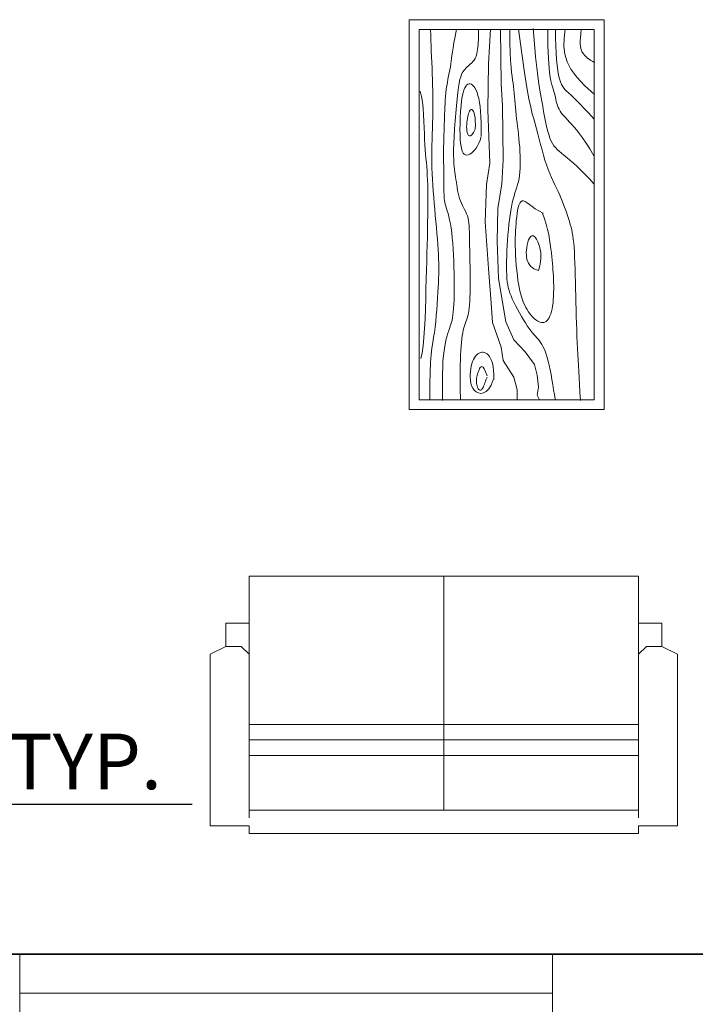
# Model space of a CAD drawing. Units: inches. Extents: x 1265 to 2734, y 1741 to 2595.
# Tile 5 of 10: x 2573 to 2634, y 1988 to 2076. Entities that reach past the tile are written whole.
import ezdxf

# ---------------------------------------------------------------- set-up
doc = ezdxf.new("R2010")
doc.units = ezdxf.units.IN
doc.header["$LTSCALE"] = 0.1
for name, color, linetype, lineweight in [('A-ANNO-DIMS', 2, 'Continuous', 18), ('A-GLAZ', 4, 'Continuous', 18), ('A-WALL', 7, 'Continuous', 35), ('Furniture', 8, 'Continuous', 15)]:
    doc.layers.add(name, color=color, linetype=linetype, lineweight=lineweight)
doc.styles.get("Standard").update_dxf_attribs({"font": 'arial.ttf', "height": 5})
doc.dimstyles.new('ISO-25', dxfattribs={"dimtxt": 5, "dimasz": 2.5, "dimexe": 1.25, "dimexo": 0.625, "dimtad": 1, "dimlunit": 3, "dimtxsty": 'Standard', "dimcen": 2.5, "dimadec": 0, "dimazin": 0, "dimtfac": 1, "dimtmove": 0, "dimatfit": 3, "dimfxl": 1, "dimarcsym": 0})

# ---------------------------------------------------------------- blocks, each defined once
blk = doc.blocks.new('WINDOW-48IN')
for p, q in [((0, 9), (0, 0)), ((48, 9), (0, 9)), ((48, 9), (48, 0)), ((48, 5.5), (0, 5.5)), ((48, 3.5), (0, 3.5)), ((0, 0), (48, 0))]:
    blk.add_line(p, q)
blk = doc.blocks.new('*D34')
at = {"layer": 'A-ANNO-DIMS', "color": 0, "lineweight": -2, "transparency": 16777216}
for p, q in [((2441.102, 2014.032), (2441.102, 2004.407)), ((2501.102, 2014.032), (2501.102, 2004.407)), ((2443.602, 2005.657), (2498.602, 2005.657)), ((2501.102, 2005.657), (2588.642, 2005.657))]:
    blk.add_line(p, q, dxfattribs=at)
at = {"layer": 'A-ANNO-DIMS', "color": 0, "lineweight": 100, "transparency": 16777216}
for points in [[(2443.602, 2006.073), (2443.602, 2005.24), (2441.102, 2005.657)], [(2498.602, 2006.073), (2498.602, 2005.24), (2501.102, 2005.657)]]:
    blk.add_solid(points, dxfattribs=at)
at = {"layer": 'Defpoints', "color": 0, "lineweight": 100, "transparency": 16777216}
for p in [(2441.102, 2014.657), (2501.102, 2014.657), (2501.102, 2005.657)]:
    blk.add_point(p, dxfattribs=at)
at = {"layer": 'A-ANNO-DIMS', "color": 0, "transparency": 16777216, "insert": (2546.122, 2008.869), "char_height": 5, "attachment_point": 5}
blk.add_mtext('DOUBLE DOOR 5\'-0" TYP.', dxfattribs=at)

msp = doc.modelspace()

# ---------------------------------------------------------------- linework, layer by layer
at = {"layer": 'A-WALL'}
msp.add_line((2514.602, 1992.157), (2679.602, 1992.157), dxfattribs=at)
at = {"layer": 'Furniture'}
for p, q in [((2608.19, 2041.186), (2608.19, 2076.268)), ((2608.19, 2076.268), (2625.731, 2076.268)), ((2625.731, 2076.268), (2625.731, 2041.186)), ((2609.067, 2042.063), (2609.067, 2075.391)), ((2609.067, 2075.391), (2624.854, 2075.391)), ((2610.115, 2075.344), (2610.119, 2074.885)), ((2612.454, 2075.404), (2612.315, 2074.746)), ((2614.432, 2075.344), (2614.421, 2074.614)), ((2615.511, 2075.404), (2615.332, 2072.285)), ((2616.411, 2075.344), (2616.471, 2070.485)), ((2617.25, 2075.344), (2617.258, 2074.223)), ((2618.03, 2075.404), (2618.322, 2073.226)), ((2619.349, 2075.464), (2619.459, 2074.082)), ((2620.668, 2075.344), (2620.682, 2073.911)), ((2621.347, 2075.424), (2621.354, 2074.634)), ((2622.227, 2075.404), (2622.126, 2074.593)), ((2623.666, 2075.404), (2623.627, 2075.005)), ((2624.854, 2075.391), (2624.854, 2042.063)), ((2610.119, 2074.885), (2610.13, 2074.409)), ((2610.13, 2074.409), (2610.146, 2073.92)), ((2612.315, 2074.746), (2612.209, 2074.2)), ((2614.421, 2074.614), (2614.39, 2074.03)), ((2621.354, 2074.634), (2621.374, 2073.913)), ((2622.126, 2074.593), (2622.108, 2073.853)), ((2623.6, 2074.659), (2623.587, 2074.36)), ((2623.627, 2075.005), (2623.6, 2074.659)), ((2610.146, 2073.92), (2610.167, 2073.421)), ((2612.131, 2073.747), (2612.074, 2073.372)), ((2612.209, 2074.2), (2612.131, 2073.747)), ((2614.342, 2073.573), (2614.279, 2073.223)), ((2614.39, 2074.03), (2614.342, 2073.573)), ((2617.258, 2074.223), (2617.28, 2073.312)), ((2619.459, 2074.082), (2619.563, 2072.929)), ((2620.682, 2073.911), (2620.722, 2072.779)), ((2621.374, 2073.913), (2621.407, 2073.259)), ((2622.108, 2073.853), (2622.192, 2073.159)), ((2623.587, 2074.36), (2623.589, 2074.101)), ((2623.589, 2074.101), (2623.607, 2073.877)), ((2623.607, 2073.877), (2623.643, 2073.681)), ((2623.643, 2073.681), (2623.697, 2073.507)), ((2623.697, 2073.507), (2623.771, 2073.349)), ((2610.167, 2073.421), (2610.19, 2072.916)), ((2610.19, 2072.916), (2610.214, 2072.406)), ((2611.998, 2072.78), (2611.968, 2072.529)), ((2612.032, 2073.055), (2611.998, 2072.78)), ((2612.074, 2073.372), (2612.032, 2073.055)), ((2614.022, 2072.618), (2613.923, 2072.5)), ((2614.116, 2072.765), (2614.022, 2072.618)), ((2614.202, 2072.96), (2614.116, 2072.765)), ((2614.279, 2073.223), (2614.202, 2072.96)), ((2617.28, 2073.312), (2617.313, 2072.581)), ((2618.322, 2073.226), (2618.572, 2071.505)), ((2619.563, 2072.929), (2619.663, 2071.97)), ((2620.722, 2072.779), (2620.782, 2071.905)), ((2621.407, 2073.259), (2621.451, 2072.671)), ((2621.451, 2072.671), (2621.505, 2072.148)), ((2622.192, 2073.159), (2622.399, 2072.487)), ((2623.771, 2073.349), (2623.865, 2073.202)), ((2623.865, 2073.202), (2623.978, 2073.065)), ((2623.978, 2073.065), (2624.105, 2072.936)), ((2624.105, 2072.936), (2624.245, 2072.815)), ((2624.245, 2072.815), (2624.394, 2072.702)), ((2624.394, 2072.702), (2624.549, 2072.597)), ((2610.214, 2072.406), (2610.238, 2071.897)), ((2610.238, 2071.897), (2610.26, 2071.39)), ((2611.843, 2071.768), (2611.789, 2071.495)), ((2611.892, 2072.032), (2611.843, 2071.768)), ((2611.934, 2072.285), (2611.892, 2072.032)), ((2611.968, 2072.529), (2611.934, 2072.285)), ((2613.212, 2071.826), (2613.123, 2071.725)), ((2613.307, 2071.922), (2613.212, 2071.826)), ((2613.406, 2072.015), (2613.307, 2071.922)), ((2613.508, 2072.107), (2613.406, 2072.015)), ((2613.612, 2072.199), (2613.508, 2072.107)), ((2613.716, 2072.293), (2613.612, 2072.199)), ((2613.82, 2072.393), (2613.716, 2072.293)), ((2613.923, 2072.5), (2613.82, 2072.393)), ((2615.332, 2072.285), (2615.272, 2068.145)), ((2617.313, 2072.581), (2617.354, 2072)), ((2617.354, 2072), (2617.4, 2071.536)), ((2619.663, 2071.97), (2619.76, 2071.174)), ((2620.782, 2071.905), (2620.856, 2071.246)), ((2621.505, 2072.148), (2621.569, 2071.688)), ((2622.399, 2072.487), (2622.75, 2071.812)), ((2622.75, 2071.812), (2623.264, 2071.11)), ((2624.549, 2072.597), (2624.707, 2072.498)), ((2624.707, 2072.498), (2624.865, 2072.405)), ((2610.26, 2071.39), (2610.279, 2070.888)), ((2610.279, 2070.888), (2610.294, 2070.392)), ((2611.676, 2070.921), (2611.62, 2070.623)), ((2611.733, 2071.212), (2611.676, 2070.921)), ((2611.789, 2071.495), (2611.733, 2071.212)), ((2612.755, 2070.879), (2612.69, 2070.568)), ((2612.821, 2071.129), (2612.755, 2070.879)), ((2612.89, 2071.327), (2612.821, 2071.129)), ((2612.963, 2071.485), (2612.89, 2071.327)), ((2613.04, 2071.614), (2612.963, 2071.485)), ((2613.123, 2071.725), (2613.04, 2071.614)), ((2617.4, 2071.536), (2617.448, 2071.16)), ((2617.448, 2071.16), (2617.496, 2070.84)), ((2618.572, 2071.505), (2618.786, 2070.171)), ((2619.76, 2071.174), (2619.853, 2070.507)), ((2620.856, 2071.246), (2620.939, 2070.76)), ((2621.569, 2071.688), (2621.642, 2071.289)), ((2621.642, 2071.289), (2621.722, 2070.95)), ((2621.722, 2070.95), (2621.81, 2070.668)), ((2623.264, 2071.11), (2623.962, 2070.356)), ((2610.294, 2070.392), (2610.306, 2069.899)), ((2611.524, 2070.005), (2611.487, 2069.688)), ((2611.569, 2070.317), (2611.524, 2070.005)), ((2611.62, 2070.623), (2611.569, 2070.317)), ((2612.627, 2070.183), (2612.563, 2069.715)), ((2612.69, 2070.568), (2612.627, 2070.183)), ((2613.189, 2070.139), (2613.107, 2069.933)), ((2613.277, 2070.293), (2613.189, 2070.139)), ((2613.371, 2070.401), (2613.277, 2070.293)), ((2613.47, 2070.467), (2613.371, 2070.401)), ((2613.573, 2070.495), (2613.47, 2070.467)), ((2613.679, 2070.49), (2613.573, 2070.495)), ((2613.788, 2070.451), (2613.679, 2070.49)), ((2613.896, 2070.377), (2613.788, 2070.451)), ((2614.003, 2070.268), (2613.896, 2070.377)), ((2614.106, 2070.123), (2614.003, 2070.268)), ((2614.204, 2069.94), (2614.106, 2070.123)), ((2616.471, 2070.485), (2616.591, 2068.505)), ((2617.496, 2070.84), (2617.54, 2070.545)), ((2617.54, 2070.545), (2617.578, 2070.25)), ((2617.578, 2070.25), (2617.611, 2069.949)), ((2618.786, 2070.171), (2618.97, 2069.156)), ((2619.853, 2070.507), (2619.943, 2069.936)), ((2620.939, 2070.76), (2621.024, 2070.405)), ((2621.024, 2070.405), (2621.107, 2070.137)), ((2621.107, 2070.137), (2621.183, 2069.915)), ((2621.81, 2070.668), (2621.905, 2070.437)), ((2621.905, 2070.437), (2622.005, 2070.247)), ((2622.005, 2070.247), (2622.113, 2070.091)), ((2622.113, 2070.091), (2622.226, 2069.959)), ((2622.226, 2069.959), (2622.344, 2069.843)), ((2623.962, 2070.356), (2624.865, 2069.525)), ((2609.156, 2069.825), (2609.275, 2069.365)), ((2609.275, 2069.365), (2609.365, 2068.85)), ((2610.306, 2069.899), (2610.314, 2069.41)), ((2610.314, 2069.41), (2610.318, 2068.921)), ((2611.457, 2069.366), (2611.433, 2069.043)), ((2611.487, 2069.688), (2611.457, 2069.366)), ((2612.5, 2069.158), (2612.437, 2068.529)), ((2612.563, 2069.715), (2612.5, 2069.158)), ((2612.964, 2069.351), (2612.903, 2068.965)), ((2613.032, 2069.672), (2612.964, 2069.351)), ((2613.107, 2069.933), (2613.032, 2069.672)), ((2614.295, 2069.72), (2614.204, 2069.94)), ((2614.377, 2069.46), (2614.295, 2069.72)), ((2614.449, 2069.161), (2614.377, 2069.46)), ((2614.51, 2068.82), (2614.449, 2069.161)), ((2617.611, 2069.949), (2617.641, 2069.643)), ((2617.641, 2069.643), (2617.667, 2069.331)), ((2617.667, 2069.331), (2617.693, 2069.015)), ((2618.97, 2069.156), (2619.13, 2068.39)), ((2619.943, 2069.936), (2620.032, 2069.428)), ((2620.032, 2069.428), (2620.118, 2068.95)), ((2621.183, 2069.915), (2621.246, 2069.703)), ((2621.246, 2069.703), (2621.299, 2069.494)), ((2621.299, 2069.494), (2621.345, 2069.29)), ((2621.345, 2069.29), (2621.388, 2069.091)), ((2621.388, 2069.091), (2621.431, 2068.899)), ((2622.344, 2069.843), (2622.468, 2069.734)), ((2622.468, 2069.734), (2622.597, 2069.625)), ((2622.597, 2069.625), (2622.732, 2069.506)), ((2622.732, 2069.506), (2622.885, 2069.364)), ((2622.885, 2069.364), (2623.067, 2069.187)), ((2623.067, 2069.187), (2623.29, 2068.963)), ((2609.365, 2068.85), (2609.431, 2068.296)), ((2609.431, 2068.296), (2609.478, 2067.717)), ((2610.318, 2068.434), (2610.314, 2067.945)), ((2610.318, 2068.921), (2610.318, 2068.434)), ((2611.399, 2068.397), (2611.386, 2068.077)), ((2611.414, 2068.719), (2611.399, 2068.397)), ((2611.433, 2069.043), (2611.414, 2068.719)), ((2612.437, 2068.529), (2612.377, 2067.852)), ((2612.851, 2068.514), (2612.809, 2068.012)), ((2612.903, 2068.965), (2612.851, 2068.514)), ((2614.561, 2068.435), (2614.51, 2068.82)), ((2614.601, 2068.006), (2614.561, 2068.435)), ((2616.591, 2068.505), (2616.651, 2063.646)), ((2617.693, 2069.015), (2617.72, 2068.693)), ((2617.72, 2068.693), (2617.748, 2068.367)), ((2617.748, 2068.367), (2617.78, 2068.035)), ((2619.13, 2068.39), (2619.271, 2067.805)), ((2620.118, 2068.95), (2620.204, 2068.475)), ((2620.204, 2068.475), (2620.29, 2068.004)), ((2621.431, 2068.899), (2621.478, 2068.713)), ((2621.478, 2068.713), (2621.533, 2068.535)), ((2621.533, 2068.535), (2621.597, 2068.365)), ((2621.597, 2068.365), (2621.676, 2068.204)), ((2621.676, 2068.204), (2621.768, 2068.05)), ((2623.29, 2068.963), (2623.567, 2068.677)), ((2623.567, 2068.677), (2623.911, 2068.318)), ((2623.911, 2068.318), (2624.332, 2067.871)), ((2609.478, 2067.717), (2609.511, 2067.13)), ((2610.305, 2067.455), (2610.292, 2066.963)), ((2610.314, 2067.945), (2610.305, 2067.455)), ((2611.364, 2067.455), (2611.353, 2067.155)), ((2611.375, 2067.763), (2611.364, 2067.455)), ((2611.386, 2068.077), (2611.375, 2067.763)), ((2612.377, 2067.852), (2612.321, 2067.151)), ((2612.778, 2067.479), (2612.758, 2066.934)), ((2612.809, 2068.012), (2612.778, 2067.479)), ((2613.424, 2067.388), (2613.395, 2067.21)), ((2613.457, 2067.554), (2613.424, 2067.388)), ((2613.493, 2067.705), (2613.457, 2067.554)), ((2613.531, 2067.838), (2613.493, 2067.705)), ((2613.572, 2067.951), (2613.531, 2067.838)), ((2613.614, 2068.043), (2613.572, 2067.951)), ((2613.659, 2068.113), (2613.614, 2068.043)), ((2613.706, 2068.159), (2613.659, 2068.113)), ((2613.756, 2068.181), (2613.706, 2068.159)), ((2613.808, 2068.176), (2613.756, 2068.181)), ((2613.863, 2068.145), (2613.808, 2068.176)), ((2613.92, 2068.085), (2613.863, 2068.145)), ((2613.976, 2067.992), (2613.92, 2068.085)), ((2614.03, 2067.859), (2613.976, 2067.992)), ((2614.076, 2067.68), (2614.03, 2067.859)), ((2614.113, 2067.452), (2614.076, 2067.68)), ((2614.137, 2067.167), (2614.113, 2067.452)), ((2614.633, 2067.53), (2614.601, 2068.006)), ((2614.655, 2067.006), (2614.633, 2067.53)), ((2615.272, 2068.145), (2615.451, 2063.346)), ((2617.78, 2068.035), (2617.816, 2067.699)), ((2617.816, 2067.699), (2617.855, 2067.358)), ((2617.855, 2067.358), (2617.897, 2067.012)), ((2619.271, 2067.805), (2619.401, 2067.332)), ((2619.401, 2067.332), (2619.524, 2066.901)), ((2620.29, 2068.004), (2620.376, 2067.542)), ((2620.376, 2067.542), (2620.464, 2067.097)), ((2621.768, 2068.05), (2621.875, 2067.897)), ((2621.875, 2067.897), (2621.996, 2067.744)), ((2621.996, 2067.744), (2622.131, 2067.587)), ((2622.131, 2067.587), (2622.282, 2067.422)), ((2622.282, 2067.422), (2622.447, 2067.246)), ((2624.332, 2067.871), (2624.845, 2067.325)), ((2609.511, 2067.13), (2609.535, 2066.55)), ((2609.535, 2066.55), (2609.555, 2065.992)), ((2610.275, 2066.468), (2610.258, 2065.969)), ((2610.292, 2066.963), (2610.275, 2066.468)), ((2611.328, 2066.558), (2611.317, 2066.249)), ((2611.341, 2066.858), (2611.328, 2066.558)), ((2611.353, 2067.155), (2611.341, 2066.858)), ((2612.272, 2066.447), (2612.232, 2065.764)), ((2612.321, 2067.151), (2612.272, 2066.447)), ((2612.758, 2066.934), (2612.752, 2066.396)), ((2613.359, 2066.834), (2613.354, 2066.644)), ((2613.354, 2066.644), (2613.36, 2066.456)), ((2613.374, 2067.024), (2613.359, 2066.834)), ((2613.36, 2066.456), (2613.378, 2066.276)), ((2613.395, 2067.21), (2613.374, 2067.024)), ((2614.132, 2066.406), (2614.144, 2066.82)), ((2614.144, 2066.82), (2614.137, 2067.167)), ((2614.668, 2066.432), (2614.655, 2067.006)), ((2614.672, 2065.806), (2614.668, 2066.432)), ((2617.897, 2067.012), (2617.94, 2066.659)), ((2617.94, 2066.659), (2617.983, 2066.301)), ((2619.524, 2066.901), (2619.645, 2066.455)), ((2619.645, 2066.455), (2619.767, 2065.991)), ((2620.464, 2067.097), (2620.555, 2066.676)), ((2620.555, 2066.676), (2620.648, 2066.284)), ((2622.447, 2067.246), (2622.627, 2067.056)), ((2622.627, 2067.056), (2622.822, 2066.846)), ((2622.822, 2066.846), (2623.034, 2066.609)), ((2623.034, 2066.609), (2623.267, 2066.332)), ((2609.555, 2065.992), (2609.575, 2065.471)), ((2610.258, 2065.969), (2610.241, 2065.468)), ((2611.297, 2065.587), (2611.289, 2065.221)), ((2611.306, 2065.928), (2611.297, 2065.587)), ((2611.317, 2066.249), (2611.306, 2065.928)), ((2612.232, 2065.764), (2612.202, 2065.126)), ((2612.752, 2066.396), (2612.76, 2065.885)), ((2612.76, 2065.885), (2612.783, 2065.418)), ((2613.378, 2066.276), (2613.409, 2066.107)), ((2613.409, 2066.107), (2613.456, 2065.963)), ((2613.456, 2065.963), (2613.519, 2065.857)), ((2613.519, 2065.857), (2613.6, 2065.805)), ((2613.6, 2065.805), (2613.7, 2065.819)), ((2613.7, 2065.819), (2613.821, 2065.914)), ((2613.821, 2065.914), (2613.965, 2066.105)), ((2613.965, 2066.105), (2614.132, 2066.406)), ((2614.574, 2065.428), (2614.672, 2065.746)), ((2617.983, 2066.301), (2618.024, 2065.936)), ((2618.024, 2065.936), (2618.064, 2065.565)), ((2618.064, 2065.565), (2618.1, 2065.186)), ((2619.767, 2065.991), (2619.89, 2065.514)), ((2620.648, 2066.284), (2620.746, 2065.928)), ((2620.746, 2065.928), (2620.848, 2065.616)), ((2620.848, 2065.616), (2620.956, 2065.35)), ((2623.267, 2066.332), (2623.521, 2066.007)), ((2623.521, 2066.007), (2623.8, 2065.622)), ((2623.8, 2065.622), (2624.105, 2065.167)), ((2609.575, 2065.471), (2609.601, 2064.999)), ((2609.601, 2064.999), (2609.63, 2064.569)), ((2610.227, 2064.964), (2610.216, 2064.458)), ((2610.241, 2065.468), (2610.227, 2064.964)), ((2611.284, 2064.826), (2611.282, 2064.398)), ((2611.289, 2065.221), (2611.284, 2064.826)), ((2612.202, 2065.126), (2612.184, 2064.556)), ((2612.783, 2065.418), (2612.823, 2065.016)), ((2612.823, 2065.016), (2612.881, 2064.693)), ((2612.881, 2064.693), (2612.954, 2064.446)), ((2614.068, 2064.516), (2614.206, 2064.693)), ((2614.206, 2064.693), (2614.338, 2064.903)), ((2614.338, 2064.903), (2614.462, 2065.147)), ((2614.462, 2065.147), (2614.574, 2065.428)), ((2618.1, 2065.186), (2618.131, 2064.8)), ((2618.131, 2064.8), (2618.156, 2064.412)), ((2619.89, 2065.514), (2620.015, 2065.032)), ((2620.015, 2065.032), (2620.143, 2064.552)), ((2620.956, 2065.35), (2621.073, 2065.125)), ((2621.073, 2065.125), (2621.201, 2064.93)), ((2621.201, 2064.93), (2621.344, 2064.757)), ((2621.344, 2064.757), (2621.504, 2064.594)), ((2624.105, 2065.167), (2624.439, 2064.632)), ((2609.63, 2064.569), (2609.662, 2064.171)), ((2609.662, 2064.171), (2609.695, 2063.793)), ((2609.695, 2063.793), (2609.729, 2063.426)), ((2610.216, 2064.458), (2610.212, 2063.948)), ((2610.212, 2063.948), (2610.215, 2063.436)), ((2611.282, 2064.398), (2611.282, 2063.945)), ((2611.282, 2063.945), (2611.284, 2063.479)), ((2612.184, 2064.556), (2612.179, 2064.071)), ((2612.179, 2064.071), (2612.187, 2063.663)), ((2612.954, 2064.446), (2613.042, 2064.268)), ((2613.042, 2064.268), (2613.143, 2064.152)), ((2613.143, 2064.152), (2613.255, 2064.091)), ((2613.255, 2064.091), (2613.377, 2064.078)), ((2613.377, 2064.078), (2613.507, 2064.105)), ((2613.507, 2064.105), (2613.643, 2064.166)), ((2613.643, 2064.166), (2613.783, 2064.254)), ((2613.783, 2064.254), (2613.926, 2064.371)), ((2613.926, 2064.371), (2614.068, 2064.516)), ((2618.156, 2064.412), (2618.175, 2064.024)), ((2618.175, 2064.024), (2618.185, 2063.642)), ((2620.143, 2064.552), (2620.273, 2064.081)), ((2620.273, 2064.081), (2620.408, 2063.627)), ((2621.504, 2064.594), (2621.684, 2064.434)), ((2621.684, 2064.434), (2621.887, 2064.266)), ((2621.887, 2064.266), (2622.117, 2064.081)), ((2622.117, 2064.081), (2622.375, 2063.871)), ((2622.375, 2063.871), (2622.659, 2063.631)), ((2624.439, 2064.632), (2624.805, 2064.006)), ((2609.729, 2063.426), (2609.761, 2063.057)), ((2609.761, 2063.057), (2609.79, 2062.678)), ((2610.215, 2063.436), (2610.227, 2062.921)), ((2610.227, 2062.921), (2610.247, 2062.403)), ((2611.284, 2063.479), (2611.287, 2063.011)), ((2611.287, 2063.011), (2611.291, 2062.553)), ((2612.187, 2063.663), (2612.204, 2063.32)), ((2612.204, 2063.32), (2612.229, 2063.029)), ((2612.229, 2063.029), (2612.259, 2062.776)), ((2615.451, 2063.346), (2615.152, 2061.427)), ((2616.651, 2063.646), (2616.531, 2061.486)), ((2618.176, 2062.912), (2618.154, 2062.573)), ((2618.185, 2063.27), (2618.176, 2062.912)), ((2618.185, 2063.642), (2618.185, 2063.27)), ((2620.408, 2063.627), (2620.548, 2063.196)), ((2620.548, 2063.196), (2620.693, 2062.795)), ((2622.659, 2063.631), (2622.968, 2063.362)), ((2622.968, 2063.362), (2623.3, 2063.059)), ((2623.3, 2063.059), (2623.652, 2062.723)), ((2609.79, 2062.678), (2609.815, 2062.276)), ((2609.815, 2062.276), (2609.835, 2061.844)), ((2610.247, 2062.403), (2610.275, 2061.881)), ((2611.291, 2062.553), (2611.296, 2062.115)), ((2611.296, 2062.115), (2611.3, 2061.709)), ((2612.259, 2062.776), (2612.293, 2062.548)), ((2612.293, 2062.548), (2612.329, 2062.333)), ((2612.329, 2062.333), (2612.364, 2062.116)), ((2612.364, 2062.116), (2612.396, 2061.889)), ((2618.12, 2062.256), (2618.072, 2061.965)), ((2618.154, 2062.573), (2618.12, 2062.256)), ((2620.693, 2062.795), (2620.842, 2062.42)), ((2620.842, 2062.42), (2620.994, 2062.067)), ((2620.994, 2062.067), (2621.146, 2061.733)), ((2623.652, 2062.723), (2624.021, 2062.35)), ((2624.021, 2062.35), (2624.406, 2061.938)), ((2609.835, 2061.844), (2609.85, 2061.38)), ((2609.85, 2061.38), (2609.859, 2060.886)), ((2610.275, 2061.881), (2610.309, 2061.355)), ((2610.309, 2061.355), (2610.348, 2060.825)), ((2611.3, 2061.709), (2611.304, 2061.347)), ((2611.304, 2061.347), (2611.308, 2061.035)), ((2612.396, 2061.889), (2612.428, 2061.65)), ((2612.428, 2061.65), (2612.461, 2061.405)), ((2612.461, 2061.405), (2612.497, 2061.155)), ((2612.497, 2061.155), (2612.539, 2060.905)), ((2615.152, 2061.427), (2615.032, 2058.067)), ((2616.531, 2061.486), (2616.171, 2059.267)), ((2617.867, 2061.185), (2617.787, 2060.934)), ((2617.943, 2061.436), (2617.867, 2061.185)), ((2618.012, 2061.694), (2617.943, 2061.436)), ((2618.072, 2061.965), (2618.012, 2061.694)), ((2621.146, 2061.733), (2621.299, 2061.412)), ((2621.299, 2061.412), (2621.449, 2061.1)), ((2621.449, 2061.1), (2621.596, 2060.793)), ((2624.406, 2061.938), (2624.805, 2061.486)), ((2609.859, 2060.886), (2609.864, 2060.363)), ((2609.864, 2060.363), (2609.865, 2059.812)), ((2610.348, 2060.825), (2610.391, 2060.291)), ((2610.391, 2060.291), (2610.437, 2059.752)), ((2611.308, 2061.035), (2611.312, 2060.769)), ((2611.312, 2060.769), (2611.318, 2060.541)), ((2611.318, 2060.541), (2611.328, 2060.342)), ((2611.328, 2060.342), (2611.343, 2060.163)), ((2612.539, 2060.905), (2612.587, 2060.658)), ((2612.587, 2060.658), (2612.645, 2060.418)), ((2612.645, 2060.418), (2612.713, 2060.187)), ((2617.621, 2060.401), (2617.54, 2060.107)), ((2617.704, 2060.675), (2617.621, 2060.401)), ((2617.787, 2060.934), (2617.704, 2060.675)), ((2621.596, 2060.793), (2621.737, 2060.487)), ((2621.737, 2060.487), (2621.873, 2060.178)), ((2609.865, 2059.812), (2609.862, 2059.235)), ((2610.437, 2059.752), (2610.485, 2059.207)), ((2611.343, 2060.163), (2611.365, 2059.997)), ((2611.365, 2059.997), (2611.395, 2059.834)), ((2611.395, 2059.834), (2611.434, 2059.667)), ((2611.434, 2059.667), (2611.484, 2059.487)), ((2611.484, 2059.487), (2611.544, 2059.29)), ((2612.713, 2060.187), (2612.794, 2059.968)), ((2612.794, 2059.968), (2612.885, 2059.76)), ((2612.885, 2059.76), (2612.981, 2059.56)), ((2612.981, 2059.56), (2613.079, 2059.367)), ((2613.079, 2059.367), (2613.176, 2059.177)), ((2617.392, 2059.438), (2617.326, 2059.066)), ((2617.464, 2059.786), (2617.392, 2059.438)), ((2617.54, 2060.107), (2617.464, 2059.786)), ((2617.945, 2059.097), (2617.999, 2059.356)), ((2617.999, 2059.356), (2618.064, 2059.58)), ((2618.064, 2059.58), (2618.143, 2059.761)), ((2618.143, 2059.761), (2618.235, 2059.889)), ((2618.235, 2059.889), (2618.345, 2059.957)), ((2618.345, 2059.957), (2618.472, 2059.957)), ((2618.472, 2059.957), (2618.623, 2059.897)), ((2618.623, 2059.897), (2618.801, 2059.788)), ((2618.801, 2059.788), (2619.01, 2059.638)), ((2619.01, 2059.638), (2619.255, 2059.459)), ((2619.255, 2059.459), (2619.54, 2059.261)), ((2621.873, 2060.178), (2622.001, 2059.867)), ((2622.001, 2059.867), (2622.123, 2059.558)), ((2622.123, 2059.558), (2622.237, 2059.252)), ((2609.855, 2058.633), (2609.845, 2058.007)), ((2609.862, 2059.235), (2609.855, 2058.633)), ((2610.485, 2059.207), (2610.534, 2058.658)), ((2610.534, 2058.658), (2610.583, 2058.108)), ((2611.544, 2059.29), (2611.609, 2059.072)), ((2611.609, 2059.072), (2611.679, 2058.829)), ((2611.679, 2058.829), (2611.751, 2058.557)), ((2611.751, 2058.557), (2611.822, 2058.252)), ((2613.176, 2059.177), (2613.268, 2058.989)), ((2613.268, 2058.989), (2613.352, 2058.8)), ((2613.352, 2058.8), (2613.423, 2058.607)), ((2613.423, 2058.607), (2613.479, 2058.408)), ((2616.171, 2059.267), (2616.111, 2056.327)), ((2617.264, 2058.672), (2617.208, 2058.257)), ((2617.326, 2059.066), (2617.264, 2058.672)), ((2617.83, 2058.207), (2617.862, 2058.514)), ((2617.862, 2058.514), (2617.9, 2058.814)), ((2617.9, 2058.814), (2617.945, 2059.097)), ((2619.54, 2059.261), (2619.869, 2059.053)), ((2619.869, 2059.053), (2620.248, 2058.847)), ((2620.188, 2058.847), (2620.373, 2058.354)), ((2622.237, 2059.252), (2622.344, 2058.951)), ((2622.344, 2058.951), (2622.443, 2058.659)), ((2622.443, 2058.659), (2622.534, 2058.377)), ((2609.845, 2058.007), (2609.833, 2057.358)), ((2610.583, 2058.108), (2610.63, 2057.565)), ((2610.63, 2057.565), (2610.676, 2057.032)), ((2611.822, 2058.252), (2611.891, 2057.91)), ((2611.891, 2057.91), (2611.954, 2057.527)), ((2613.479, 2058.408), (2613.521, 2058.199)), ((2613.521, 2058.199), (2613.552, 2057.973)), ((2613.552, 2057.973), (2613.574, 2057.726)), ((2613.574, 2057.726), (2613.589, 2057.452)), ((2615.032, 2058.067), (2615.332, 2053.868)), ((2617.156, 2057.823), (2617.111, 2057.373)), ((2617.208, 2058.257), (2617.156, 2057.823)), ((2617.759, 2057.276), (2617.778, 2057.591)), ((2617.778, 2057.591), (2617.802, 2057.9)), ((2617.802, 2057.9), (2617.83, 2058.207)), ((2620.373, 2058.354), (2620.525, 2057.868)), ((2620.525, 2057.868), (2620.649, 2057.391)), ((2622.534, 2058.377), (2622.617, 2058.107)), ((2622.617, 2058.107), (2622.691, 2057.851)), ((2622.691, 2057.851), (2622.758, 2057.601)), ((2622.758, 2057.601), (2622.817, 2057.35)), ((2609.818, 2056.685), (2609.8, 2055.986)), ((2609.833, 2057.358), (2609.818, 2056.685)), ((2610.676, 2057.032), (2610.718, 2056.517)), ((2611.954, 2057.527), (2612.01, 2057.101)), ((2612.01, 2057.101), (2612.059, 2056.637)), ((2613.589, 2057.452), (2613.599, 2057.146)), ((2613.599, 2057.146), (2613.606, 2056.803)), ((2613.606, 2056.803), (2613.613, 2056.417)), ((2617.07, 2056.907), (2617.036, 2056.429)), ((2617.111, 2057.373), (2617.07, 2056.907)), ((2617.737, 2056.615), (2617.745, 2056.952)), ((2617.745, 2056.952), (2617.759, 2057.276)), ((2619.083, 2056.707), (2619.011, 2056.597)), ((2619.158, 2056.779), (2619.083, 2056.707)), ((2619.232, 2056.817), (2619.158, 2056.779)), ((2619.306, 2056.825), (2619.232, 2056.817)), ((2619.379, 2056.807), (2619.306, 2056.825)), ((2619.449, 2056.766), (2619.379, 2056.807)), ((2619.516, 2056.704), (2619.449, 2056.766)), ((2619.581, 2056.621), (2619.516, 2056.704)), ((2620.649, 2057.391), (2620.749, 2056.928)), ((2620.749, 2056.928), (2620.828, 2056.482)), ((2622.817, 2057.35), (2622.87, 2057.09)), ((2622.87, 2057.09), (2622.917, 2056.811)), ((2622.917, 2056.811), (2622.958, 2056.507)), ((2609.8, 2055.986), (2609.782, 2055.258)), ((2610.718, 2056.517), (2610.756, 2056.024)), ((2610.756, 2056.024), (2610.789, 2055.559)), ((2612.059, 2056.637), (2612.102, 2056.143)), ((2612.102, 2056.143), (2612.137, 2055.625)), ((2613.613, 2056.417), (2613.621, 2055.987)), ((2613.621, 2055.987), (2613.631, 2055.518)), ((2616.111, 2056.327), (2616.231, 2052.968)), ((2617.007, 2055.946), (2616.984, 2055.463)), ((2617.036, 2056.429), (2617.007, 2055.946)), ((2617.734, 2056.261), (2617.737, 2056.615)), ((2617.739, 2055.887), (2617.734, 2056.261)), ((2617.75, 2055.488), (2617.739, 2055.887)), ((2618.814, 2056.002), (2618.762, 2055.707)), ((2618.875, 2056.248), (2618.814, 2056.002)), ((2618.941, 2056.445), (2618.875, 2056.248)), ((2619.011, 2056.597), (2618.941, 2056.445)), ((2619.644, 2056.52), (2619.581, 2056.621)), ((2619.706, 2056.401), (2619.644, 2056.52)), ((2619.766, 2056.265), (2619.706, 2056.401)), ((2619.825, 2056.113), (2619.766, 2056.265)), ((2619.883, 2055.947), (2619.825, 2056.113)), ((2619.94, 2055.768), (2619.883, 2055.947)), ((2620.828, 2056.482), (2620.89, 2056.057)), ((2620.89, 2056.057), (2620.941, 2055.656)), ((2622.958, 2056.507), (2622.994, 2056.168)), ((2622.994, 2056.168), (2623.026, 2055.787)), ((2623.026, 2055.787), (2623.055, 2055.358)), ((2609.782, 2055.258), (2609.761, 2054.501)), ((2610.789, 2055.559), (2610.815, 2055.128)), ((2610.815, 2055.128), (2610.833, 2054.733)), ((2612.137, 2055.625), (2612.167, 2055.091)), ((2612.167, 2055.091), (2612.191, 2054.549)), ((2613.631, 2055.518), (2613.64, 2055.023)), ((2613.64, 2055.023), (2613.65, 2054.51)), ((2616.968, 2054.988), (2616.958, 2054.528)), ((2616.984, 2055.463), (2616.968, 2054.988)), ((2617.769, 2055.062), (2617.75, 2055.488)), ((2617.795, 2054.618), (2617.769, 2055.062)), ((2618.762, 2055.707), (2618.73, 2055.377)), ((2618.73, 2055.377), (2618.735, 2055.031)), ((2618.735, 2055.031), (2618.791, 2054.686)), ((2619.991, 2055.569), (2619.94, 2055.768)), ((2620.029, 2055.347), (2619.991, 2055.569)), ((2620.049, 2055.095), (2620.029, 2055.347)), ((2620.045, 2054.809), (2620.049, 2055.095)), ((2620.941, 2055.656), (2620.983, 2055.283)), ((2620.983, 2055.283), (2621.02, 2054.939)), ((2621.02, 2054.939), (2621.053, 2054.622)), ((2623.055, 2055.358), (2623.079, 2054.884)), ((2609.761, 2054.501), (2609.74, 2053.712)), ((2610.833, 2054.733), (2610.845, 2054.367)), ((2610.845, 2054.367), (2610.85, 2054.019)), ((2610.85, 2054.019), (2610.85, 2053.679)), ((2612.191, 2054.549), (2612.21, 2054.006)), ((2613.65, 2054.51), (2613.659, 2053.991)), ((2616.958, 2054.528), (2616.955, 2054.09)), ((2616.955, 2054.09), (2616.959, 2053.681)), ((2617.829, 2054.161), (2617.795, 2054.618)), ((2617.871, 2053.702), (2617.829, 2054.161)), ((2618.791, 2054.686), (2618.913, 2054.361)), ((2618.913, 2054.361), (2619.117, 2054.074)), ((2619.117, 2054.074), (2619.417, 2053.844)), ((2619.829, 2053.688), (2619.941, 2054.111)), ((2619.941, 2054.111), (2620.011, 2054.482)), ((2620.011, 2054.482), (2620.045, 2054.809)), ((2621.053, 2054.622), (2621.083, 2054.324)), ((2621.083, 2054.324), (2621.108, 2054.04)), ((2621.108, 2054.04), (2621.13, 2053.764)), ((2623.079, 2054.884), (2623.102, 2054.371)), ((2623.102, 2054.371), (2623.121, 2053.825)), ((2609.74, 2053.712), (2609.718, 2052.89)), ((2610.843, 2053.335), (2610.831, 2052.978)), ((2610.85, 2053.679), (2610.843, 2053.335)), ((2612.21, 2054.006), (2612.224, 2053.468)), ((2612.224, 2053.468), (2612.233, 2052.943)), ((2613.659, 2053.991), (2613.666, 2053.476)), ((2613.666, 2053.476), (2613.671, 2052.975)), ((2615.332, 2053.868), (2615.571, 2050.748)), ((2616.959, 2053.681), (2616.97, 2053.308)), ((2616.97, 2053.308), (2616.989, 2052.976)), ((2617.921, 2053.247), (2617.871, 2053.702)), ((2617.979, 2052.806), (2617.921, 2053.247)), ((2619.417, 2053.844), (2619.829, 2053.688)), ((2621.13, 2053.764), (2621.149, 2053.491)), ((2621.149, 2053.491), (2621.165, 2053.214)), ((2621.165, 2053.214), (2621.178, 2052.928)), ((2623.121, 2053.825), (2623.139, 2053.252)), ((2623.139, 2053.252), (2623.156, 2052.658)), ((2609.718, 2052.89), (2609.695, 2052.033)), ((2610.815, 2052.596), (2610.795, 2052.178)), ((2610.831, 2052.978), (2610.815, 2052.596)), ((2612.233, 2052.943), (2612.237, 2052.435)), ((2612.237, 2052.435), (2612.236, 2051.948)), ((2613.671, 2052.975), (2613.673, 2052.498)), ((2613.673, 2052.498), (2613.671, 2052.054)), ((2616.231, 2052.968), (2616.891, 2049.069)), ((2616.989, 2052.976), (2617.018, 2052.678)), ((2617.018, 2052.678), (2617.057, 2052.406)), ((2617.057, 2052.406), (2617.108, 2052.152)), ((2618.045, 2052.387), (2617.979, 2052.806)), ((2618.12, 2051.998), (2618.045, 2052.387)), ((2621.178, 2052.928), (2621.187, 2052.629)), ((2621.187, 2052.629), (2621.193, 2052.319)), ((2621.193, 2052.319), (2621.194, 2052.004)), ((2623.156, 2052.658), (2623.171, 2052.048)), ((2609.695, 2052.033), (2609.672, 2051.143)), ((2610.77, 2051.718), (2610.741, 2051.223)), ((2610.795, 2052.178), (2610.77, 2051.718)), ((2612.23, 2051.486), (2612.219, 2051.053)), ((2612.236, 2051.948), (2612.23, 2051.486)), ((2613.665, 2051.643), (2613.654, 2051.265)), ((2613.671, 2052.054), (2613.665, 2051.643)), ((2617.108, 2052.152), (2617.173, 2051.906)), ((2617.173, 2051.906), (2617.254, 2051.661)), ((2617.254, 2051.661), (2617.353, 2051.408)), ((2617.353, 2051.408), (2617.47, 2051.138)), ((2618.202, 2051.646), (2618.12, 2051.998)), ((2618.292, 2051.329), (2618.202, 2051.646)), ((2621.179, 2051.373), (2621.161, 2051.068)), ((2621.19, 2051.687), (2621.179, 2051.373)), ((2621.194, 2052.004), (2621.19, 2051.687)), ((2623.171, 2052.048), (2623.186, 2051.428)), ((2623.186, 2051.428), (2623.201, 2050.805)), ((2609.672, 2051.143), (2609.646, 2050.238)), ((2610.708, 2050.704), (2610.669, 2050.17)), ((2610.741, 2051.223), (2610.708, 2050.704)), ((2612.203, 2050.653), (2612.181, 2050.29)), ((2612.219, 2051.053), (2612.203, 2050.653)), ((2613.616, 2050.601), (2613.588, 2050.313)), ((2613.638, 2050.918), (2613.616, 2050.601)), ((2613.654, 2051.265), (2613.638, 2050.918)), ((2615.571, 2050.748), (2615.691, 2049.009)), ((2617.47, 2051.138), (2617.607, 2050.846)), ((2617.607, 2050.846), (2617.761, 2050.535)), ((2617.761, 2050.535), (2617.928, 2050.214)), ((2618.387, 2051.045), (2618.292, 2051.329)), ((2618.487, 2050.791), (2618.387, 2051.045)), ((2618.589, 2050.564), (2618.487, 2050.791)), ((2618.693, 2050.362), (2618.589, 2050.564)), ((2621.098, 2050.498), (2621.051, 2050.243)), ((2621.134, 2050.775), (2621.098, 2050.498)), ((2621.161, 2051.068), (2621.134, 2050.775)), ((2623.201, 2050.805), (2623.217, 2050.181)), ((2609.646, 2050.238), (2609.612, 2049.342)), ((2610.624, 2049.634), (2610.573, 2049.105)), ((2610.669, 2050.17), (2610.624, 2049.634)), ((2612.121, 2049.69), (2612.083, 2049.447)), ((2612.154, 2049.968), (2612.121, 2049.69)), ((2612.181, 2050.29), (2612.154, 2049.968)), ((2613.464, 2049.609), (2613.41, 2049.418)), ((2613.513, 2049.818), (2613.464, 2049.609)), ((2613.554, 2050.053), (2613.513, 2049.818)), ((2613.588, 2050.313), (2613.554, 2050.053)), ((2617.928, 2050.214), (2618.103, 2049.89)), ((2618.103, 2049.89), (2618.284, 2049.57)), ((2618.797, 2050.181), (2618.693, 2050.362)), ((2618.899, 2050.018), (2618.797, 2050.181)), ((2618.999, 2049.873), (2618.899, 2050.018)), ((2619.097, 2049.741), (2618.999, 2049.873)), ((2619.193, 2049.624), (2619.097, 2049.741)), ((2619.289, 2049.519), (2619.193, 2049.624)), ((2620.859, 2049.614), (2620.78, 2049.451)), ((2620.931, 2049.8), (2620.859, 2049.614)), ((2620.996, 2050.01), (2620.931, 2049.8)), ((2621.051, 2050.243), (2620.996, 2050.01)), ((2623.217, 2050.181), (2623.233, 2049.562)), ((2609.612, 2049.342), (2609.568, 2048.476)), ((2610.573, 2049.105), (2610.515, 2048.595)), ((2611.936, 2048.855), (2611.877, 2048.675)), ((2611.99, 2049.039), (2611.936, 2048.855)), ((2612.039, 2049.233), (2611.99, 2049.039)), ((2612.083, 2049.447), (2612.039, 2049.233)), ((2613.167, 2048.719), (2613.108, 2048.528)), ((2613.228, 2048.897), (2613.167, 2048.719)), ((2613.29, 2049.069), (2613.228, 2048.897)), ((2613.352, 2049.24), (2613.29, 2049.069)), ((2613.41, 2049.418), (2613.352, 2049.24)), ((2615.691, 2049.009), (2616.471, 2046.789)), ((2616.891, 2049.069), (2617.61, 2047.449)), ((2618.284, 2049.57), (2618.466, 2049.261)), ((2618.466, 2049.261), (2618.646, 2048.972)), ((2618.646, 2048.972), (2618.819, 2048.709)), ((2618.819, 2048.709), (2618.983, 2048.477)), ((2619.385, 2049.425), (2619.289, 2049.519)), ((2619.481, 2049.341), (2619.385, 2049.425)), ((2619.579, 2049.266), (2619.481, 2049.341)), ((2619.679, 2049.199), (2619.579, 2049.266)), ((2619.781, 2049.139), (2619.679, 2049.199)), ((2619.886, 2049.088), (2619.781, 2049.139)), ((2619.991, 2049.049), (2619.886, 2049.088)), ((2620.097, 2049.024), (2619.991, 2049.049)), ((2620.203, 2049.016), (2620.097, 2049.024)), ((2620.307, 2049.027), (2620.203, 2049.016)), ((2620.409, 2049.061), (2620.307, 2049.027)), ((2620.508, 2049.119), (2620.409, 2049.061)), ((2620.603, 2049.203), (2620.508, 2049.119)), ((2620.694, 2049.315), (2620.603, 2049.203)), ((2620.78, 2049.451), (2620.694, 2049.315)), ((2623.233, 2049.562), (2623.249, 2048.951)), ((2623.249, 2048.951), (2623.267, 2048.351)), ((2609.568, 2048.476), (2609.51, 2047.663)), ((2610.45, 2048.114), (2610.377, 2047.664)), ((2610.515, 2048.595), (2610.45, 2048.114)), ((2611.595, 2047.818), (2611.52, 2047.539)), ((2611.671, 2048.067), (2611.595, 2047.818)), ((2611.744, 2048.289), (2611.671, 2048.067)), ((2611.813, 2048.489), (2611.744, 2048.289)), ((2611.877, 2048.675), (2611.813, 2048.489)), ((2612.959, 2047.824), (2612.92, 2047.536)), ((2613.003, 2048.085), (2612.959, 2047.824)), ((2613.053, 2048.319), (2613.003, 2048.085)), ((2613.108, 2048.528), (2613.053, 2048.319)), ((2618.983, 2048.477), (2619.137, 2048.274)), ((2619.137, 2048.274), (2619.282, 2048.094)), ((2619.282, 2048.094), (2619.42, 2047.933)), ((2619.42, 2047.933), (2619.551, 2047.783)), ((2623.267, 2048.351), (2623.287, 2047.768)), ((2609.434, 2046.926), (2609.337, 2046.287)), ((2609.51, 2047.663), (2609.434, 2046.926)), ((2610.302, 2047.212), (2610.228, 2046.715)), ((2610.377, 2047.664), (2610.302, 2047.212)), ((2611.447, 2047.225), (2611.378, 2046.872)), ((2611.52, 2047.539), (2611.447, 2047.225)), ((2612.886, 2047.22), (2612.856, 2046.873)), ((2612.92, 2047.536), (2612.886, 2047.22)), ((2617.61, 2047.449), (2618.629, 2046.369)), ((2619.551, 2047.783), (2619.675, 2047.642)), ((2619.675, 2047.642), (2619.794, 2047.502)), ((2619.794, 2047.502), (2619.908, 2047.359)), ((2619.908, 2047.359), (2620.019, 2047.208)), ((2620.019, 2047.208), (2620.126, 2047.044)), ((2620.126, 2047.044), (2620.23, 2046.863)), ((2623.287, 2047.768), (2623.308, 2047.204)), ((2623.308, 2047.204), (2623.331, 2046.664)), ((2609.337, 2046.287), (2609.216, 2045.769)), ((2610.161, 2046.134), (2610.105, 2045.424)), ((2610.228, 2046.715), (2610.161, 2046.134)), ((2611.265, 2046.033), (2611.224, 2045.539)), ((2611.317, 2046.476), (2611.265, 2046.033)), ((2611.378, 2046.872), (2611.317, 2046.476)), ((2612.81, 2046.087), (2612.793, 2045.644)), ((2612.831, 2046.496), (2612.81, 2046.087)), ((2612.856, 2046.873), (2612.831, 2046.496)), ((2614.263, 2046.095), (2614.16, 2045.98)), ((2614.372, 2046.189), (2614.263, 2046.095)), ((2614.487, 2046.26), (2614.372, 2046.189)), ((2614.606, 2046.308), (2614.487, 2046.26)), ((2614.728, 2046.333), (2614.606, 2046.308)), ((2614.85, 2046.333), (2614.728, 2046.333)), ((2614.972, 2046.308), (2614.85, 2046.333)), ((2615.091, 2046.258), (2614.972, 2046.308)), ((2615.207, 2046.182), (2615.091, 2046.258)), ((2615.317, 2046.079), (2615.207, 2046.182)), ((2615.42, 2045.948), (2615.317, 2046.079)), ((2616.471, 2046.789), (2616.651, 2045.589)), ((2618.629, 2046.369), (2619.469, 2045.229)), ((2620.23, 2046.863), (2620.33, 2046.66)), ((2620.33, 2046.66), (2620.427, 2046.431)), ((2620.427, 2046.431), (2620.522, 2046.172)), ((2620.522, 2046.172), (2620.614, 2045.877)), ((2623.331, 2046.664), (2623.357, 2046.148)), ((2623.357, 2046.148), (2623.385, 2045.645)), ((2610.105, 2045.424), (2610.066, 2044.545)), ((2611.224, 2045.539), (2611.197, 2044.995)), ((2612.78, 2045.17), (2612.771, 2044.676)), ((2612.793, 2045.644), (2612.78, 2045.17)), ((2613.828, 2045.31), (2613.77, 2045.094)), ((2613.897, 2045.508), (2613.828, 2045.31)), ((2613.976, 2045.685), (2613.897, 2045.508)), ((2614.064, 2045.843), (2613.976, 2045.685)), ((2614.16, 2045.98), (2614.064, 2045.843)), ((2615.514, 2045.786), (2615.42, 2045.948)), ((2615.598, 2045.585), (2615.514, 2045.786)), ((2615.671, 2045.343), (2615.598, 2045.585)), ((2615.73, 2045.053), (2615.671, 2045.343)), ((2616.651, 2045.589), (2617.61, 2044.089)), ((2619.469, 2045.229), (2619.709, 2044.269)), ((2620.614, 2045.877), (2620.703, 2045.544)), ((2620.703, 2045.544), (2620.79, 2045.17)), ((2620.79, 2045.17), (2620.874, 2044.761)), ((2623.385, 2045.645), (2623.415, 2045.137)), ((2610.066, 2044.545), (2610.047, 2043.454)), ((2611.182, 2044.424), (2611.175, 2043.853)), ((2611.197, 2044.995), (2611.182, 2044.424)), ((2612.771, 2044.676), (2612.766, 2044.174)), ((2613.669, 2044.345), (2613.668, 2044.079)), ((2613.688, 2044.608), (2613.669, 2044.345)), ((2613.723, 2044.859), (2613.688, 2044.608)), ((2613.77, 2045.094), (2613.723, 2044.859)), ((2614.335, 2044.367), (2614.3, 2044.241)), ((2614.376, 2044.493), (2614.335, 2044.367)), ((2614.422, 2044.619), (2614.376, 2044.493)), ((2614.472, 2044.744), (2614.422, 2044.619)), ((2614.527, 2044.867), (2614.472, 2044.744)), ((2614.588, 2044.971), (2614.527, 2044.867)), ((2614.657, 2045.039), (2614.588, 2044.971)), ((2614.737, 2045.052), (2614.657, 2045.039)), ((2614.83, 2044.994), (2614.737, 2045.052)), ((2614.939, 2044.846), (2614.83, 2044.994)), ((2615.065, 2044.591), (2614.939, 2044.846)), ((2615.212, 2044.209), (2615.065, 2044.591)), ((2615.774, 2044.711), (2615.73, 2045.053)), ((2615.802, 2044.312), (2615.774, 2044.711)), ((2615.811, 2043.85), (2615.802, 2044.312)), ((2619.709, 2044.269), (2619.829, 2043.19)), ((2620.874, 2044.761), (2620.956, 2044.327)), ((2620.956, 2044.327), (2621.036, 2043.878)), ((2623.415, 2045.137), (2623.448, 2044.61)), ((2623.448, 2044.61), (2623.483, 2044.047)), ((2610.047, 2043.454), (2610.055, 2042.11)), ((2611.175, 2043.853), (2611.176, 2043.311)), ((2612.766, 2044.174), (2612.766, 2043.68)), ((2612.766, 2043.68), (2612.77, 2043.207)), ((2613.668, 2044.079), (2613.688, 2043.815)), ((2613.688, 2043.815), (2613.733, 2043.56)), ((2613.733, 2043.56), (2613.806, 2043.321)), ((2614.237, 2043.87), (2614.232, 2043.75)), ((2614.232, 2043.75), (2614.237, 2043.631)), ((2614.25, 2043.993), (2614.237, 2043.87)), ((2614.237, 2043.631), (2614.25, 2043.516)), ((2614.271, 2044.117), (2614.25, 2043.993)), ((2614.25, 2043.516), (2614.27, 2043.406)), ((2614.27, 2043.406), (2614.297, 2043.303)), ((2614.3, 2044.241), (2614.271, 2044.117)), ((2614.91, 2043.343), (2614.952, 2043.462)), ((2614.952, 2043.462), (2614.995, 2043.588)), ((2614.995, 2043.588), (2615.041, 2043.718)), ((2615.041, 2043.718), (2615.092, 2043.847)), ((2615.092, 2043.847), (2615.148, 2043.972)), ((2615.148, 2043.972), (2615.212, 2044.089)), ((2615.341, 2043.034), (2615.557, 2043.378)), ((2615.557, 2043.378), (2615.751, 2043.85)), ((2617.61, 2044.089), (2617.91, 2042.95)), ((2621.036, 2043.878), (2621.113, 2043.422)), ((2621.113, 2043.422), (2621.187, 2042.969)), ((2623.483, 2044.047), (2623.522, 2043.434)), ((2623.522, 2043.434), (2623.562, 2042.753)), ((2611.176, 2043.311), (2611.18, 2042.826)), ((2611.18, 2042.826), (2611.186, 2042.425)), ((2612.77, 2043.207), (2612.779, 2042.768)), ((2612.779, 2042.768), (2612.794, 2042.378)), ((2613.806, 2043.321), (2613.91, 2043.106)), ((2613.91, 2043.106), (2614.047, 2042.92)), ((2614.047, 2042.92), (2614.22, 2042.771)), ((2614.22, 2042.771), (2614.421, 2042.673)), ((2614.297, 2043.303), (2614.33, 2043.21)), ((2614.33, 2043.21), (2614.367, 2043.127)), ((2614.367, 2043.127), (2614.408, 2043.056)), ((2614.408, 2043.056), (2614.452, 2043)), ((2614.421, 2042.673), (2614.642, 2042.637)), ((2614.452, 2043), (2614.498, 2042.959)), ((2614.498, 2042.959), (2614.545, 2042.934)), ((2614.545, 2042.934), (2614.593, 2042.926)), ((2614.593, 2042.926), (2614.641, 2042.935)), ((2614.641, 2042.935), (2614.689, 2042.96)), ((2614.642, 2042.637), (2614.875, 2042.676)), ((2614.689, 2042.96), (2614.737, 2043.002)), ((2614.737, 2043.002), (2614.783, 2043.062)), ((2614.783, 2043.062), (2614.827, 2043.14)), ((2614.827, 2043.14), (2614.869, 2043.234)), ((2614.869, 2043.234), (2614.91, 2043.343)), ((2614.875, 2042.676), (2615.111, 2042.804)), ((2615.111, 2042.804), (2615.341, 2043.034)), ((2617.91, 2042.95), (2617.91, 2042.05)), ((2619.829, 2043.19), (2619.709, 2042.47)), ((2621.187, 2042.969), (2621.259, 2042.529)), ((2621.259, 2042.529), (2621.328, 2042.11)), ((2623.562, 2042.753), (2623.606, 2041.99)), ((2624.854, 2042.063), (2609.067, 2042.063)), ((2611.186, 2042.425), (2611.192, 2042.137)), ((2611.192, 2042.137), (2611.194, 2041.99)), ((2612.794, 2042.378), (2612.813, 2042.05)), ((2619.709, 2042.47), (2619.888, 2042.11)), ((2625.731, 2041.186), (2608.19, 2041.186)), ((2593.759, 2026.178), (2628.841, 2026.178)), ((2593.759, 2021.969), (2593.759, 2026.178)), ((2611.3, 2026.178), (2611.3, 2005.129)), ((2628.841, 2026.178), (2628.841, 2021.969)), ((2591.654, 2019.864), (2591.654, 2021.969)), ((2591.654, 2021.969), (2593.759, 2021.969)), ((2593.759, 2021.969), (2593.759, 2019.162)), ((2628.841, 2021.969), (2628.841, 2019.162)), ((2628.841, 2021.969), (2630.946, 2021.969)), ((2630.946, 2021.969), (2630.946, 2019.864)), ((2590.251, 2019.162), (2591.654, 2019.864)), ((2591.654, 2019.864), (2593.058, 2019.864)), ((2593.058, 2019.864), (2593.759, 2019.162)), ((2629.543, 2019.864), (2628.841, 2019.162)), ((2630.946, 2019.864), (2629.543, 2019.864)), ((2630.946, 2019.864), (2632.349, 2019.162)), ((2590.251, 2003.726), (2590.251, 2019.162)), ((2593.759, 2019.162), (2593.759, 2004.428)), ((2628.841, 2019.162), (2628.841, 2004.428)), ((2632.349, 2019.162), (2632.349, 2003.726)), ((2593.759, 2012.847), (2628.841, 2012.847)), ((2593.759, 2011.444), (2628.841, 2011.444)), ((2593.759, 2010.041), (2628.841, 2010.041)), ((2628.841, 2005.129), (2593.759, 2005.129)), ((2593.759, 2003.726), (2590.251, 2003.726)), ((2593.759, 2003.024), (2593.759, 2003.726)), ((2632.349, 2003.726), (2628.841, 2003.726)), ((2628.841, 2003.726), (2628.841, 2003.024)), ((2628.841, 2003.024), (2593.759, 2003.024))]:
    msp.add_line(p, q, dxfattribs=at)

# ---------------------------------------------------------------- block references
at = {"layer": 'A-GLAZ'}
msp.add_blockref('WINDOW-48IN', (2573.102, 1983.157), dxfattribs=at)

# ---------------------------------------------------------------- dimensions: what is measured, and where the dimension line sits
at = {"layer": 'A-ANNO-DIMS'}
dim = msp.add_linear_dim(base=(2501.102, 2005.657), p1=(2441.102, 2014.657), p2=(2501.102, 2014.657), text='DOUBLE DOOR <> TYP.', dimstyle='ISO-25', override={"dimdec": 1, "dimlfac": 1, "dimrnd": 0, "dimzin": 1, "dimdsep": 46, "dimlunit": 4, "dimfrac": 2}, dxfattribs=at)
dim.commit()
dim.dimension.update_dxf_attribs({"geometry": '*D34', "text_midpoint": (2546.122, 2008.869)})

doc.saveas('drawing.dxf')
